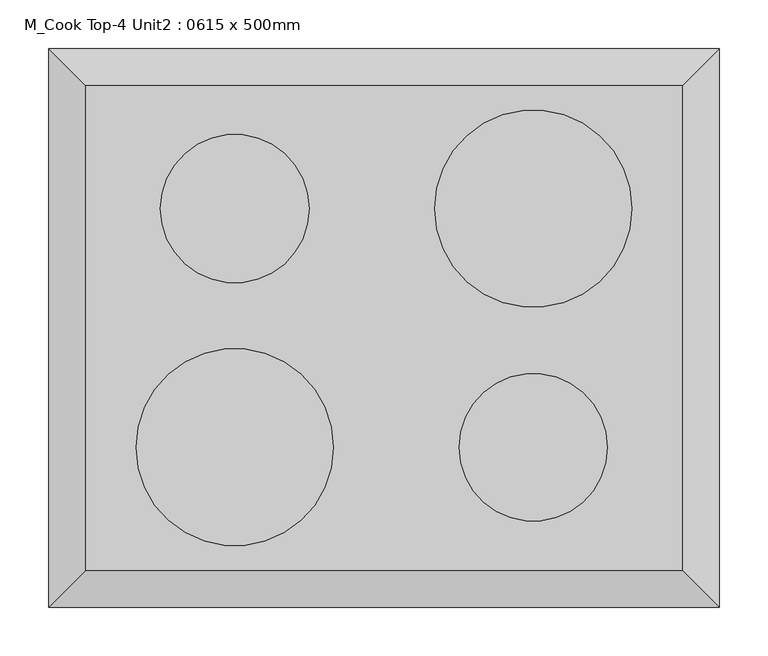
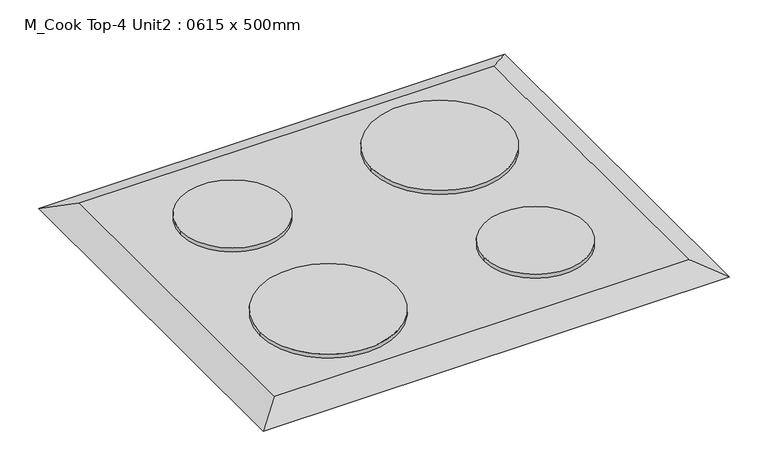
"""IFC4 building model written with IfcOpenShell, lengths in millimetres: proxy geometry, M_Cook Top-4 Unit2 : 0615 x 500mm."""

from ifc_helpers import new_model, si_unit, point, frame, frame_2d, origin, place, context, project, spatial, circle_curve, trimmed, segment, composite_curve, outline, extrude, faceted_brep, source, transform, mapped, element, save


def m_cook_top_4_unit2_0615_x_500mm_249f3515(model_context):
    return source(origin(), model_context, "Body", "SolidModel", [
        faceted_brep([(307.5, 250.0, 918.0), (-307.5, 250.0, 918.0), (-307.5, -250.0, 918.0), (307.5, -250.0, 918.0), (345.6, 288.1, 900.0), (345.6, -288.1, 900.0), (-345.6, -288.1, 900.0), (-345.6, 288.1, 900.0)], [[[0, 1, 2, 3]], [[4, 5, 6, 7]], [[4, 7, 1, 0]], [[7, 6, 2, 1]], [[6, 5, 3, 2]], [[5, 4, 0, 3]]]),
        extrude(outline(composite_curve([segment(trimmed(circle_curve(frame_2d((153.75, -123.0)), 76.2), [point((77.55, -123.0))], [point((229.95, -123.0))], False, "CARTESIAN"), True, "CONTINUOUS"), segment(trimmed(circle_curve(frame_2d((153.75, -123.0)), 76.2), [point((229.95, -123.0))], [point((77.55, -123.0))], False, "CARTESIAN"), True, "CONTINUOUS")], self_intersect=False)), frame((0.0, 0.0, 918.0), z_axis=(0.0, 0.0, 1.0), x_axis=(1.0, 0.0, 0.0)), (0.0, 0.0, 1.0), 6.35),
        extrude(outline(composite_curve([segment(trimmed(circle_curve(frame_2d((153.75, 123.0)), 101.6), [point((52.15, 123.0))], [point((255.35, 123.0))], False, "CARTESIAN"), True, "CONTINUOUS"), segment(trimmed(circle_curve(frame_2d((153.75, 123.0)), 101.6), [point((255.35, 123.0))], [point((52.15, 123.0))], False, "CARTESIAN"), True, "CONTINUOUS")], self_intersect=False)), frame((0.0, 0.0, 918.0), z_axis=(0.0, 0.0, 1.0), x_axis=(1.0, 0.0, 0.0)), (0.0, 0.0, 1.0), 6.35),
        extrude(outline(composite_curve([segment(trimmed(circle_curve(frame_2d((-153.75, 123.0)), 76.59), [point((-230.34, 123.0))], [point((-77.16, 123.0))], False, "CARTESIAN"), True, "CONTINUOUS"), segment(trimmed(circle_curve(frame_2d((-153.75, 123.0)), 76.59), [point((-77.16, 123.0))], [point((-230.34, 123.0))], False, "CARTESIAN"), True, "CONTINUOUS")], self_intersect=False)), frame((0.0, 0.0, 918.0), z_axis=(0.0, 0.0, 1.0), x_axis=(1.0, 0.0, 0.0)), (0.0, 0.0, 1.0), 6.35),
        extrude(outline(composite_curve([segment(trimmed(circle_curve(frame_2d((-153.75, -123.0)), 101.6), [point((-52.15, -123.0))], [point((-255.35, -123.0))], False, "CARTESIAN"), True, "CONTINUOUS"), segment(trimmed(circle_curve(frame_2d((-153.75, -123.0)), 101.6), [point((-255.35, -123.0))], [point((-52.15, -123.0))], False, "CARTESIAN"), True, "CONTINUOUS")], self_intersect=False)), frame((0.0, 0.0, 918.0), z_axis=(0.0, 0.0, 1.0), x_axis=(1.0, 0.0, 0.0)), (0.0, 0.0, 1.0), 6.35),
    ])


if __name__ == "__main__":
    model = new_model("IFC4")
    model_context = context("Model", 3, world=origin())
    ifc_project = project(units=[si_unit("LENGTHUNIT", "METRE", prefix="MILLI")], contexts=[model_context])
    site = spatial("IfcSite", under=ifc_project)
    building = spatial("IfcBuilding", under=site)
    placement = place(None, origin())
    m_cook_top_4_unit2_0615_x_500mm_shape = m_cook_top_4_unit2_0615_x_500mm_249f3515(model_context)
    element("IfcBuildingElementProxy", 1, Name="M_Cook Top-4 Unit2 : 0615 x 500mm", ObjectType="M_Cook Top-4 Unit2 : 0615 x 500mm", at=placement, inside=building, context=model_context, shape_type="MappedRepresentation", body=[
        mapped(m_cook_top_4_unit2_0615_x_500mm_shape, transform((0.0, 0.0, 0.0), x_axis=(1.0, 0.0, 0.0), y_axis=(0.0, 1.0, 0.0), z_axis=(0.0, 0.0, 1.0))),
    ])
    save(model, "model.ifc")

# Revit data of these elements
# Type "M_Cook Top-4 Unit2 : 0615 x 500mm"
#   Depth = 1' - 7.68504"
#   Width = 2' - 0.2126"
#   Burner Material = Steel, Chrome Plated
#   Cooktop Material = Steel, Polished
#   Default Elevation = 0
#   Assembly Code = ""
# Element 1 (IfcBuildingElementProxy, "M_Cook Top-4 Unit2 : 0615 x 500mm")
#   Materials on its faces: "Steel, Polished", "Steel, Chrome Plated"
# Materials
#   "Steel, Chrome Plated": class "Metal", colour RGB 244 244 244, transparency 0, Description = "Chromiuim plated steel", Cost = 0
#   "Steel, Polished": class "Metal", colour RGB 57 57 57, transparency 0, Description = "Polished steel", Cost = 0
